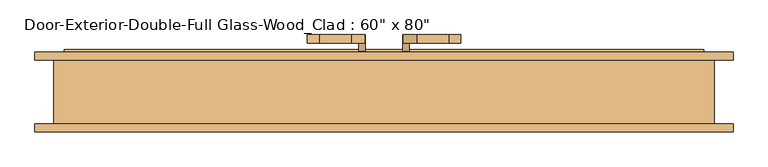
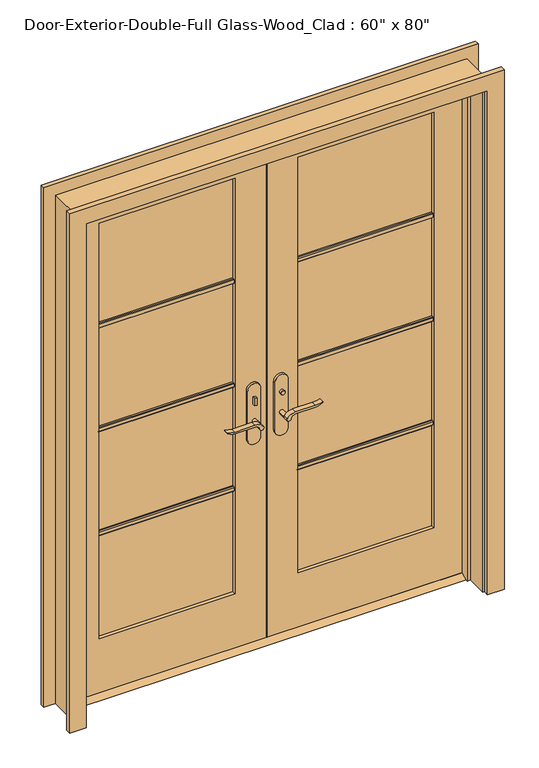
"""IFC4 building model written with IfcOpenShell, lengths in millimetres: door geometry."""

from ifc_helpers import new_model, si_unit, point, frame, frame_2d, origin, place, context, project, spatial, polyline, circle_curve, trimmed, segment, composite_curve, outline, extrude, faceted_brep, source, transform, mapped, element, save


def door_94998e6c(model_context):
    return source(origin(), model_context, "Body", "SolidModel", [
        extrude(outline(polyline([(38.1, 12.7), (73.025, 12.7), (98.425, 0.0), (12.7, 0.0), (38.1, 12.7)])), frame((-762.0, 0.0, 0.0), z_axis=(1.0, 0.0, 0.0), x_axis=(0.0, 1.0, 0.0)), (0.0, 0.0, 1.0), 1524.0),
        extrude(outline(polyline([(-47.4019111, 18.1), (-57.4019111, 18.1), (-57.4019111, 28.1), (-47.4019111, 28.1), (-47.4019111, 18.1)])), frame((0.0, 0.0, 981.9), z_axis=(0.0, 0.0, 1.0), x_axis=(1.0, 0.0, 0.0)), (0.0, 0.0, 1.0), 30.0),
        extrude(outline(composite_curve([segment(trimmed(circle_curve(frame_2d((996.9, -52.4019111)), 8.0), [point((996.9, -60.4019111))], [point((996.9, -44.4019111))], False, "CARTESIAN"), True, "CONTINUOUS"), segment(trimmed(circle_curve(frame_2d((996.9, -52.4019111)), 8.0), [point((996.9, -44.4019111))], [point((996.9, -60.4019111))], False, "CARTESIAN"), True, "CONTINUOUS")], self_intersect=False)), frame((0.0, 83.025, 0.0), z_axis=(0.0, 1.0, 0.0), x_axis=(0.0, 0.0, 1.0)), (0.0, 0.0, 1.0), 10.0),
        extrude(outline(composite_curve([segment(trimmed(circle_curve(frame_2d((897.1555521, -76.0694241)), 37.2832219), [point((919.0523287, -45.8937749))], [point((934.4, -77.7693445))], False, "CARTESIAN"), True, "CONTINUOUS"), segment(polyline([(934.4, -77.7693445), (934.4, -154.045502)]), True, "CONTINUOUS"), segment(trimmed(circle_curve(frame_2d((1017.6850638, -153.9791202)), 83.2850902), [point((934.4, -154.045502))], [point((939.4, -182.4019111))], True, "CARTESIAN"), True, "CONTINUOUS"), segment(polyline([(939.4, -182.4019111), (936.6135558, -182.4019111)]), True, "CONTINUOUS"), segment(trimmed(circle_curve(frame_2d((986.6709207, -150.4622499)), 59.3791355), [point((936.6135558, -182.4019111))], [point((927.4, -154.045502))], False, "CARTESIAN"), True, "CONTINUOUS"), segment(polyline([(927.4, -154.045502), (927.4, -77.7881013)]), True, "CONTINUOUS"), segment(trimmed(circle_curve(frame_2d((909.2738613, -77.7881013)), 18.1261387), [point((927.4, -77.7881013))], [point((914.4, -60.4019111))], True, "CARTESIAN"), True, "CONTINUOUS"), segment(trimmed(circle_curve(frame_2d((914.4, -52.4019111)), 8.0), [point((914.4, -60.4019111))], [point((919.0523287, -45.8937749))], False, "CARTESIAN"), True, "CONTINUOUS")], self_intersect=False)), frame((0.0, -21.9, 0.0), z_axis=(0.0, 1.0, 0.0), x_axis=(0.0, 0.0, 1.0)), (0.0, 0.0, 1.0), 20.0),
        extrude(outline(composite_curve([segment(trimmed(circle_curve(frame_2d((914.4, -52.4019111)), 8.0), [point((914.3999903, -60.4019111))], [point((919.0523287, -45.8937749))], False, "CARTESIAN"), True, "CONTINUOUS"), segment(trimmed(circle_curve(frame_2d((897.1555521, -76.0694241)), 37.2832219), [point((919.0523287, -45.8937749))], [point((934.4, -77.7693445))], False, "CARTESIAN"), True, "CONTINUOUS"), segment(polyline([(934.4, -77.7693445), (934.4, -154.045502)]), True, "CONTINUOUS"), segment(trimmed(circle_curve(frame_2d((1017.6850638, -153.9791202)), 83.2850902), [point((934.4, -154.045502))], [point((939.4, -182.4019111))], True, "CARTESIAN"), True, "CONTINUOUS"), segment(polyline([(939.4, -182.4019111), (936.6135558, -182.4019111)]), True, "CONTINUOUS"), segment(trimmed(circle_curve(frame_2d((986.6709207, -150.4622499)), 59.3791355), [point((936.6135558, -182.4019111))], [point((927.4, -154.045502))], False, "CARTESIAN"), True, "CONTINUOUS"), segment(polyline([(927.4, -154.045502), (927.4, -77.788099)]), True, "CONTINUOUS"), segment(trimmed(circle_curve(frame_2d((909.2738682, -77.788099)), 18.1261318), [point((927.4, -77.788099))], [point((914.3999903, -60.4019111))], True, "CARTESIAN"), True, "CONTINUOUS")], self_intersect=False)), frame((0.0, 113.025, 0.0), z_axis=(0.0, 1.0, 0.0), x_axis=(0.0, 0.0, 1.0)), (0.0, 0.0, 1.0), 20.0),
        extrude(outline(composite_curve([segment(trimmed(circle_curve(frame_2d((914.4, -52.4019111)), 8.0), [point((914.4, -60.4019111))], [point((914.4, -44.4019111))], False, "CARTESIAN"), True, "CONTINUOUS"), segment(trimmed(circle_curve(frame_2d((914.4, -52.4019111)), 8.0), [point((914.4, -44.4019111))], [point((914.4, -60.4019111))], False, "CARTESIAN"), True, "CONTINUOUS")], self_intersect=False)), frame((0.0, -1.9, 0.0), z_axis=(0.0, 1.0, 0.0), x_axis=(0.0, 0.0, 1.0)), (0.0, 0.0, 1.0), 30.0),
        extrude(outline(composite_curve([segment(trimmed(circle_curve(frame_2d((914.4, -52.4019111)), 8.0), [point((914.4, -60.4019111))], [point((914.4, -44.4019111))], False, "CARTESIAN"), True, "CONTINUOUS"), segment(trimmed(circle_curve(frame_2d((914.4, -52.4019111)), 8.0), [point((914.4, -44.4019111))], [point((914.4, -60.4019111))], False, "CARTESIAN"), True, "CONTINUOUS")], self_intersect=False)), frame((0.0, 83.025, 0.0), z_axis=(0.0, 1.0, 0.0), x_axis=(0.0, 0.0, 1.0)), (0.0, 0.0, 1.0), 30.0),
        extrude(outline(composite_curve([segment(polyline([(844.4, -27.4019111), (1039.4, -27.4019111)]), True, "CONTINUOUS"), segment(trimmed(circle_curve(frame_2d((1039.4, -52.4019111)), 25.0), [point((1039.4, -27.4019111))], [point((1039.4, -77.4019111))], False, "CARTESIAN"), True, "CONTINUOUS"), segment(polyline([(1039.4, -77.4019111), (844.4, -77.4019111)]), True, "CONTINUOUS"), segment(trimmed(circle_curve(frame_2d((844.4, -52.4019111)), 25.0), [point((844.4, -77.4019111))], [point((844.4, -27.4019111))], False, "CARTESIAN"), True, "CONTINUOUS")], self_intersect=False)), frame((0.0, 28.1, 0.0), z_axis=(0.0, 1.0, 0.0), x_axis=(0.0, 0.0, 1.0)), (0.0, 0.0, 1.0), 10.0),
        extrude(outline(composite_curve([segment(polyline([(844.4, -27.4019111), (1039.4, -27.4019111)]), True, "CONTINUOUS"), segment(trimmed(circle_curve(frame_2d((1039.4, -52.4019111)), 25.0), [point((1039.4, -27.4019111))], [point((1039.4, -77.4019111))], False, "CARTESIAN"), True, "CONTINUOUS"), segment(polyline([(1039.4, -77.4019111), (844.4, -77.4019111)]), True, "CONTINUOUS"), segment(trimmed(circle_curve(frame_2d((844.4, -52.4019111)), 25.0), [point((844.4, -77.4019111))], [point((844.4, -27.4019111))], False, "CARTESIAN"), True, "CONTINUOUS")], self_intersect=False)), frame((0.0, 73.025, 0.0), z_axis=(0.0, 1.0, 0.0), x_axis=(0.0, 0.0, 1.0)), (0.0, 0.0, 1.0), 10.0),
        extrude(outline(polyline([(47.3875, 93.025), (57.3875, 93.025), (57.3875, 83.025), (47.3875, 83.025), (47.3875, 93.025)])), frame((0.0, 0.0, 981.9), z_axis=(0.0, 0.0, 1.0), x_axis=(1.0, 0.0, 0.0)), (0.0, 0.0, 1.0), 30.0),
        extrude(outline(composite_curve([segment(trimmed(circle_curve(frame_2d((996.9, 52.3875)), 8.0), [point((996.9, 60.3875))], [point((996.9, 44.3875))], False, "CARTESIAN"), True, "CONTINUOUS"), segment(trimmed(circle_curve(frame_2d((996.9, 52.3875)), 8.0), [point((996.9, 44.3875))], [point((996.9, 60.3875))], False, "CARTESIAN"), True, "CONTINUOUS")], self_intersect=False)), frame((0.0, 18.1, 0.0), z_axis=(0.0, 1.0, 0.0), x_axis=(0.0, 0.0, 1.0)), (0.0, 0.0, 1.0), 10.0),
        extrude(outline(composite_curve([segment(trimmed(circle_curve(frame_2d((914.4, 52.3875)), 8.0), [point((919.0523287, 45.8793637))], [point((914.4, 60.3875))], False, "CARTESIAN"), True, "CONTINUOUS"), segment(trimmed(circle_curve(frame_2d((909.2738613, 77.7736901)), 18.1261387), [point((914.4, 60.3875))], [point((927.4, 77.7736901))], True, "CARTESIAN"), True, "CONTINUOUS"), segment(polyline([(927.4, 77.7736901), (927.4, 154.0310909)]), True, "CONTINUOUS"), segment(trimmed(circle_curve(frame_2d((986.6709207, 150.4478388)), 59.3791355), [point((927.4, 154.0310909))], [point((936.6135558, 182.3875))], False, "CARTESIAN"), True, "CONTINUOUS"), segment(polyline([(936.6135558, 182.3875), (939.4, 182.3875)]), True, "CONTINUOUS"), segment(trimmed(circle_curve(frame_2d((1017.6850638, 153.9647091)), 83.2850902), [point((939.4, 182.3875))], [point((934.4, 154.0310909))], True, "CARTESIAN"), True, "CONTINUOUS"), segment(polyline([(934.4, 154.0310909), (934.4, 77.7549333)]), True, "CONTINUOUS"), segment(trimmed(circle_curve(frame_2d((897.1555521, 76.0550129)), 37.2832219), [point((934.4, 77.7549333))], [point((919.0523287, 45.8793637))], False, "CARTESIAN"), True, "CONTINUOUS")], self_intersect=False)), frame((0.0, 113.025, 0.0), z_axis=(0.0, 1.0, 0.0), x_axis=(0.0, 0.0, 1.0)), (0.0, 0.0, 1.0), 20.0),
        extrude(outline(composite_curve([segment(trimmed(circle_curve(frame_2d((909.2738682, 77.7736878)), 18.1261318), [point((914.3999903, 60.3875))], [point((927.4, 77.7736878))], True, "CARTESIAN"), True, "CONTINUOUS"), segment(polyline([(927.4, 77.7736878), (927.4, 154.0310909)]), True, "CONTINUOUS"), segment(trimmed(circle_curve(frame_2d((986.6709207, 150.4478388)), 59.3791355), [point((927.4, 154.0310909))], [point((936.6135558, 182.3875))], False, "CARTESIAN"), True, "CONTINUOUS"), segment(polyline([(936.6135558, 182.3875), (939.4, 182.3875)]), True, "CONTINUOUS"), segment(trimmed(circle_curve(frame_2d((1017.6850638, 153.9647091)), 83.2850902), [point((939.4, 182.3875))], [point((934.4, 154.0310909))], True, "CARTESIAN"), True, "CONTINUOUS"), segment(polyline([(934.4, 154.0310909), (934.4, 77.7549333)]), True, "CONTINUOUS"), segment(trimmed(circle_curve(frame_2d((897.1555521, 76.0550129)), 37.2832219), [point((934.4, 77.7549333))], [point((919.0523287, 45.8793637))], False, "CARTESIAN"), True, "CONTINUOUS"), segment(trimmed(circle_curve(frame_2d((914.4, 52.3875)), 8.0), [point((919.0523287, 45.8793637))], [point((914.3999903, 60.3875))], False, "CARTESIAN"), True, "CONTINUOUS")], self_intersect=False)), frame((0.0, -21.9, 0.0), z_axis=(0.0, 1.0, 0.0), x_axis=(0.0, 0.0, 1.0)), (0.0, 0.0, 1.0), 20.0),
        extrude(outline(composite_curve([segment(trimmed(circle_curve(frame_2d((914.4, 52.3875)), 8.0), [point((914.4, 60.3875))], [point((914.4, 44.3875))], False, "CARTESIAN"), True, "CONTINUOUS"), segment(trimmed(circle_curve(frame_2d((914.4, 52.3875)), 8.0), [point((914.4, 44.3875))], [point((914.4, 60.3875))], False, "CARTESIAN"), True, "CONTINUOUS")], self_intersect=False)), frame((0.0, 83.025, 0.0), z_axis=(0.0, 1.0, 0.0), x_axis=(0.0, 0.0, 1.0)), (0.0, 0.0, 1.0), 30.0),
        extrude(outline(composite_curve([segment(trimmed(circle_curve(frame_2d((914.4, 52.3875)), 8.0), [point((914.4, 60.3875))], [point((914.4, 44.3875))], False, "CARTESIAN"), True, "CONTINUOUS"), segment(trimmed(circle_curve(frame_2d((914.4, 52.3875)), 8.0), [point((914.4, 44.3875))], [point((914.4, 60.3875))], False, "CARTESIAN"), True, "CONTINUOUS")], self_intersect=False)), frame((0.0, -1.9, 0.0), z_axis=(0.0, 1.0, 0.0), x_axis=(0.0, 0.0, 1.0)), (0.0, 0.0, 1.0), 30.0),
        extrude(outline(composite_curve([segment(trimmed(circle_curve(frame_2d((844.4, 52.3875)), 25.0), [point((844.4, 27.3875))], [point((844.4, 77.3875))], False, "CARTESIAN"), True, "CONTINUOUS"), segment(polyline([(844.4, 77.3875), (1039.4, 77.3875)]), True, "CONTINUOUS"), segment(trimmed(circle_curve(frame_2d((1039.4, 52.3875)), 25.0), [point((1039.4, 77.3875))], [point((1039.4, 27.3875))], False, "CARTESIAN"), True, "CONTINUOUS"), segment(polyline([(1039.4, 27.3875), (844.4, 27.3875)]), True, "CONTINUOUS")], self_intersect=False)), frame((0.0, 73.025, 0.0), z_axis=(0.0, 1.0, 0.0), x_axis=(0.0, 0.0, 1.0)), (0.0, 0.0, 1.0), 10.0),
        extrude(outline(composite_curve([segment(trimmed(circle_curve(frame_2d((844.4, 52.3875)), 25.0), [point((844.4, 27.3875))], [point((844.4, 77.3875))], False, "CARTESIAN"), True, "CONTINUOUS"), segment(polyline([(844.4, 77.3875), (1039.4, 77.3875)]), True, "CONTINUOUS"), segment(trimmed(circle_curve(frame_2d((1039.4, 52.3875)), 25.0), [point((1039.4, 77.3875))], [point((1039.4, 27.3875))], False, "CARTESIAN"), True, "CONTINUOUS"), segment(polyline([(1039.4, 27.3875), (844.4, 27.3875)]), True, "CONTINUOUS")], self_intersect=False)), frame((0.0, 28.1, 0.0), z_axis=(0.0, 1.0, 0.0), x_axis=(0.0, 0.0, 1.0)), (0.0, 0.0, 1.0), 10.0),
        extrude(outline(polyline([(52.07, 1502.171875), (52.07, 1483.121875), (45.72, 1483.121875), (42.545, 1486.296875), (42.545, 1498.996875), (45.72, 1502.171875), (52.07, 1502.171875)])), frame((120.65, 0.0, 0.0), z_axis=(1.0, 0.0, 0.0), x_axis=(0.0, 1.0, 0.0)), (0.0, 0.0, 1.0), 520.7),
        extrude(outline(polyline([(52.07, 1081.88125), (52.07, 1062.83125), (45.72, 1062.83125), (42.545, 1066.00625), (42.545, 1078.70625), (45.72, 1081.88125), (52.07, 1081.88125)])), frame((120.65, 0.0, 0.0), z_axis=(1.0, 0.0, 0.0), x_axis=(0.0, 1.0, 0.0)), (0.0, 0.0, 1.0), 520.7),
        extrude(outline(polyline([(52.07, 661.590625), (52.07, 642.540625), (45.72, 642.540625), (42.545, 645.715625), (42.545, 658.415625), (45.72, 661.590625), (52.07, 661.590625)])), frame((120.65, 0.0, 0.0), z_axis=(1.0, 0.0, 0.0), x_axis=(0.0, 1.0, 0.0)), (0.0, 0.0, 1.0), 520.7),
        extrude(outline(polyline([(59.055, 1502.171875), (65.405, 1502.171875), (68.58, 1498.996875), (68.58, 1486.296875), (65.405, 1483.121875), (59.055, 1483.121875), (59.055, 1502.171875)])), frame((-641.35, 0.0, 0.0), z_axis=(1.0, 0.0, 0.0), x_axis=(0.0, 1.0, 0.0)), (0.0, 0.0, 1.0), 520.7),
        extrude(outline(polyline([(59.055, 1081.88125), (65.405, 1081.88125), (68.58, 1078.70625), (68.58, 1066.00625), (65.405, 1062.83125), (59.055, 1062.83125), (59.055, 1081.88125)])), frame((-641.35, 0.0, 0.0), z_axis=(1.0, 0.0, 0.0), x_axis=(0.0, 1.0, 0.0)), (0.0, 0.0, 1.0), 520.7),
        extrude(outline(polyline([(59.055, 661.590625), (65.405, 661.590625), (68.58, 658.415625), (68.58, 645.715625), (65.405, 642.540625), (59.055, 642.540625), (59.055, 661.590625)])), frame((-641.35, 0.0, 0.0), z_axis=(1.0, 0.0, 0.0), x_axis=(0.0, 1.0, 0.0)), (0.0, 0.0, 1.0), 520.7),
        extrude(outline(polyline([(59.055, 1502.171875), (65.405, 1502.171875), (68.58, 1498.996875), (68.58, 1486.296875), (65.405, 1483.121875), (59.055, 1483.121875), (59.055, 1502.171875)])), frame((120.65, 0.0, 0.0), z_axis=(1.0, 0.0, 0.0), x_axis=(0.0, 1.0, 0.0)), (0.0, 0.0, 1.0), 520.7),
        extrude(outline(polyline([(59.055, 1081.88125), (65.405, 1081.88125), (68.58, 1078.70625), (68.58, 1066.00625), (65.405, 1062.83125), (59.055, 1062.83125), (59.055, 1081.88125)])), frame((120.65, 0.0, 0.0), z_axis=(1.0, 0.0, 0.0), x_axis=(0.0, 1.0, 0.0)), (0.0, 0.0, 1.0), 520.7),
        extrude(outline(polyline([(59.055, 661.590625), (65.405, 661.590625), (68.58, 658.415625), (68.58, 645.715625), (65.405, 642.540625), (59.055, 642.540625), (59.055, 661.590625)])), frame((120.65, 0.0, 0.0), z_axis=(1.0, 0.0, 0.0), x_axis=(0.0, 1.0, 0.0)), (0.0, 0.0, 1.0), 520.7),
        extrude(outline(polyline([(52.07, 1502.171875), (52.07, 1483.121875), (45.72, 1483.121875), (42.545, 1486.296875), (42.545, 1498.996875), (45.72, 1502.171875), (52.07, 1502.171875)])), frame((-641.35, 0.0, 0.0), z_axis=(1.0, 0.0, 0.0), x_axis=(0.0, 1.0, 0.0)), (0.0, 0.0, 1.0), 520.7),
        extrude(outline(polyline([(52.07, 1081.88125), (52.07, 1062.83125), (45.72, 1062.83125), (42.545, 1066.00625), (42.545, 1078.70625), (45.72, 1081.88125), (52.07, 1081.88125)])), frame((-641.35, 0.0, 0.0), z_axis=(1.0, 0.0, 0.0), x_axis=(0.0, 1.0, 0.0)), (0.0, 0.0, 1.0), 520.7),
        extrude(outline(polyline([(52.07, 661.590625), (52.07, 642.540625), (45.72, 642.540625), (42.545, 645.715625), (42.545, 658.415625), (45.72, 661.590625), (52.07, 661.590625)])), frame((-641.35, 0.0, 0.0), z_axis=(1.0, 0.0, 0.0), x_axis=(0.0, 1.0, 0.0)), (0.0, 0.0, 1.0), 520.7),
        extrude(outline(polyline([(0.0, 768.35), (0.0, 831.85), (2101.85, 831.85), (2101.85, -831.85), (0.0, -831.85), (0.0, -768.35), (2038.35, -768.35), (2038.35, 768.35), (0.0, 768.35)])), frame((0.0, 73.025, 0.0), z_axis=(0.0, 1.0, 0.0), x_axis=(0.0, 0.0, 1.0)), (0.0, 0.0, 1.0), 19.05),
        extrude(outline(polyline([(0.0, 768.35), (0.0, 831.85), (2101.85, 831.85), (2101.85, -831.85), (0.0, -831.85), (0.0, -768.35), (2038.35, -768.35), (2038.35, 768.35), (0.0, 768.35)])), frame((0.0, -98.425, 0.0), z_axis=(0.0, 1.0, 0.0), x_axis=(0.0, 0.0, 1.0)), (0.0, 0.0, 1.0), 19.05),
        extrude(outline(polyline([(12.7, 762.0), (2032.0, 762.0), (2032.0, 1.5875), (12.7, 1.5875), (12.7, 762.0)]), holes=[polyline([(1912.9375, 120.65), (1912.9375, 641.35), (231.775, 641.35), (231.775, 120.65), (1912.9375, 120.65)])]), frame((0.0, 38.1, 0.0), z_axis=(0.0, 1.0, 0.0), x_axis=(0.0, 0.0, 1.0)), (0.0, 0.0, 1.0), 34.925),
        extrude(outline(polyline([(2032.0, -762.0), (12.7, -762.0), (12.7, -1.6019111), (2032.0, -1.6019111), (2032.0, -762.0)]), holes=[polyline([(231.775, -641.35), (1912.9375, -641.35), (1912.9375, -120.65), (231.775, -120.65), (231.775, -641.35)])]), frame((0.0, 38.1, 0.0), z_axis=(0.0, 1.0, 0.0), x_axis=(0.0, 0.0, 1.0)), (0.0, 0.0, 1.0), 34.925),
        faceted_brep([(787.4, 73.025, 0.0), (787.4, -79.375, 0.0), (762.0, -79.375, 0.0), (762.0, 3.175, 0.0), (749.3, 3.175, 0.0), (749.3, 38.1, 0.0), (762.0, 38.1, 0.0), (762.0, 73.025, 0.0), (787.4, 73.025, 2057.4), (787.4, -79.375, 2057.4), (-787.4, -79.375, 2057.4), (-787.4, -79.375, 0.0), (-762.0, -79.375, 0.0), (-762.0, -79.375, 2032.0), (762.0, -79.375, 2032.0), (762.0, 3.175, 2032.0), (-762.0, 3.175, 2032.0), (-762.0, 3.175, 0.0), (-749.3, 3.175, 0.0), (-749.3, 3.175, 2019.3), (749.3, 3.175, 2019.3), (749.3, 38.1, 2019.3), (1.5875, 38.1, 2019.3), (-1.6019111, 38.1, 2019.3), (-749.3, 38.1, 2019.3), (-749.3, 38.1, 0.0), (-762.0, 38.1, 0.0), (-762.0, 38.1, 2032.0), (-1.6019111, 38.1, 2032.0), (1.5875, 38.1, 2032.0), (762.0, 38.1, 2032.0), (762.0, 73.025, 2032.0), (1.5875, 73.025, 2032.0), (-1.6019111, 73.025, 2032.0), (-762.0, 73.025, 2032.0), (-762.0, 73.025, 0.0), (-787.4, 73.025, 0.0), (-787.4, 73.025, 2057.4)], [[[0, 1, 2, 3, 4, 5, 6, 7]], [[1, 0, 8, 9]], [[2, 1, 9, 10, 11, 12, 13, 14]], [[3, 2, 14, 15]], [[4, 3, 15, 16, 17, 18, 19, 20]], [[5, 4, 20, 21]], [[6, 5, 21, 22, 23, 24, 25, 26, 27, 28, 29, 30]], [[7, 6, 30, 31]], [[0, 7, 31, 32, 33, 34, 35, 36, 37, 8]], [[9, 8, 37, 10]], [[14, 13, 16, 15]], [[20, 19, 24, 23, 22, 21]], [[31, 30, 29, 28, 27, 34, 33, 32]], [[12, 11, 36, 35, 26, 25, 18, 17]], [[11, 10, 37, 36]], [[13, 12, 17, 16]], [[19, 18, 25, 24]], [[27, 26, 35, 34]]]),
        extrude(outline(polyline([(641.35, 52.07), (120.65, 52.07), (120.65, 59.055), (641.35, 59.055), (641.35, 52.07)])), frame((0.0, 0.0, 231.775), z_axis=(0.0, 0.0, 1.0), x_axis=(1.0, 0.0, 0.0)), (0.0, 0.0, 1.0), 1681.1625),
        extrude(outline(polyline([(-120.65, 52.07), (-641.35, 52.07), (-641.35, 59.055), (-120.65, 59.055), (-120.65, 52.07)])), frame((0.0, 0.0, 231.775), z_axis=(0.0, 0.0, 1.0), x_axis=(1.0, 0.0, 0.0)), (0.0, 0.0, 1.0), 1681.1625),
    ])


if __name__ == "__main__":
    model = new_model("IFC4")
    model_context = context("Model", 3, world=origin())
    ifc_project = project(units=[si_unit("LENGTHUNIT", "METRE", prefix="MILLI")], contexts=[model_context])
    site = spatial("IfcSite", under=ifc_project)
    building = spatial("IfcBuilding", under=site)
    placement = place(None, origin())
    door_shape = door_94998e6c(model_context)
    element("IfcDoor", 1, ObjectType="Door-Exterior-Double-Full Glass-Wood_Clad : 60\" x 80\"", at=placement, inside=building, context=model_context, shape_type="MappedRepresentation", body=[
        mapped(door_shape, transform((0.0, 0.0, 0.0), x_axis=(1.0, 0.0, 0.0), y_axis=(0.0, 1.0, 0.0), z_axis=(0.0, 0.0, 1.0))),
    ])
    save(model, "model.ifc")

# Revit data of these elements
# Type "Door-Exterior-Double-Full Glass-Wood_Clad : 60\" x 80\""
#   Type Mark = "9"
#   Assembly Code = "B2030100"
#   Analytic Construction = "French door, wood frame with double glass"
#   Top Rail = 0' - 4 11/16"
#   Threshold Offset [instance default] = 0' - 0 1/2"
#   Thickness = 0' - 1 3/8"
#   Thermal Resistance (R) = 1.9158 (h·ft²·°F)/BTU
#   Swing Angle [instance default] = 90.00°
#   Stiles = 0' - 4 3/4"
#   Rough Width = 5' - 2"
#   Rough Height = 6' - 9"
#   Panel Width = 2' - 6"
#   Door Offset [instance default] = 0' - 0"
#   Height = 6' - 8"
#   Width = 5' - 0"
#   Heat Transfer Coefficient (U) = 0.5220 BTU/(h·ft²·°F)
#   Bottom Rail = 0' - 9 1/8"
#   Exterior Trim [instance default] = yes
#   Threshold [instance default] = yes
#   Show Grill [instance default] = yes
#   Function = 1
#   Trim Material = Cherry
#   Threshold Material = Cherry
#   Panel Material = Cherry
#   Glazing = Glass
#   Frame Material = Cherry
#   Door Handle Material = Aluminum
#   Visual Light Transmittance = 0
#   Solar Heat Gain Coefficient = 0
#   Wall Closure = (empty or 0)
#   Construction Type = (empty or 0)
# Element 1 (IfcDoor, "Door-Exterior-Double-Full Glass-Wood_Clad : 60\" x 80\"")
#   Materials on its faces: "Cherry", "Aluminum", "Glass"
# Materials
#   "Cherry": class "Wood", colour RGB 226 177 128, transparency 0, Description = "Prunus Serotina", Cost = 0
#   "Glass": class "Glass", colour RGB 0 128 192, transparency 0.75, Description = "Soda Lime Glass", Cost = 0
#   "Aluminum": class "Metal", colour RGB 247 247 247, transparency 0, Description = "Aluminum 6061", Cost = 0
